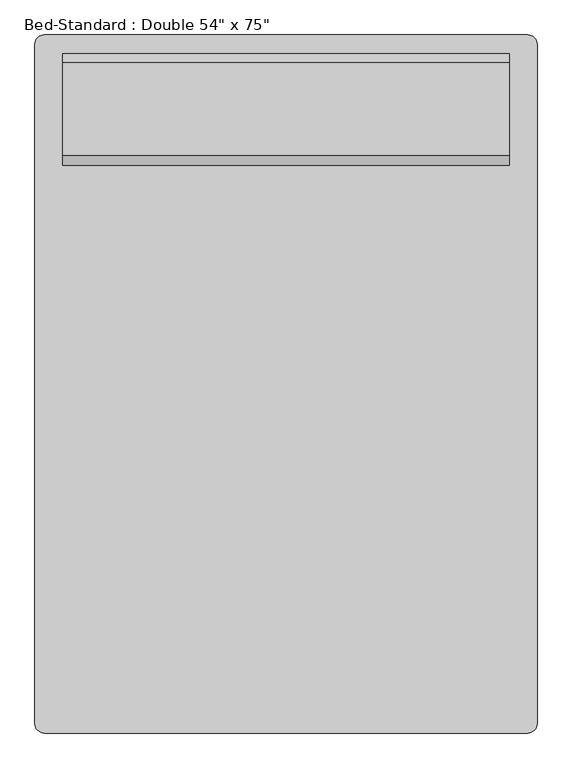
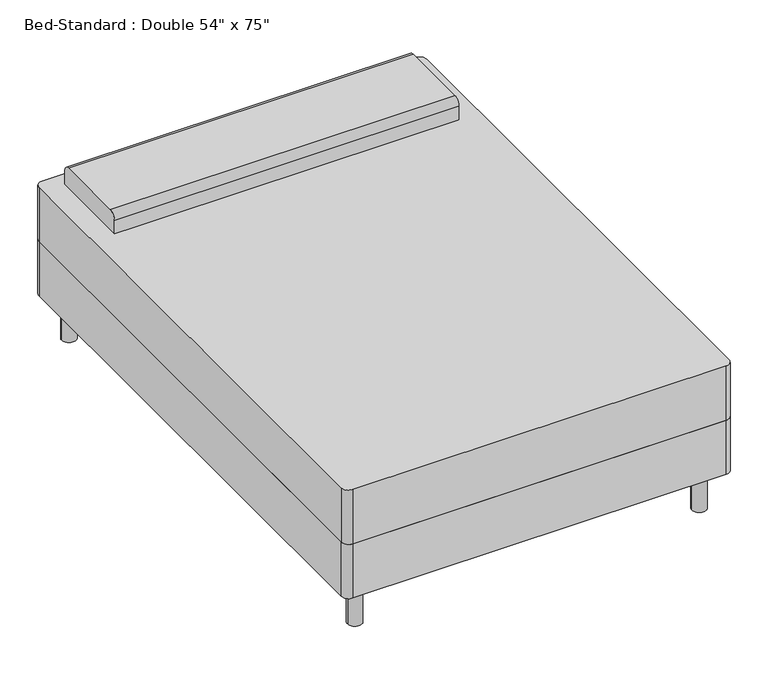
"""IFC4 building model written with IfcOpenShell, lengths in millimetres: furniture geometry."""

from ifc_helpers import new_model, si_unit, point, frame, frame_2d, origin, origin_with_axes, place, context, project, spatial, polyline, circle_curve, trimmed, segment, composite_curve, outline, extrude, source, transform, mapped, element, save


def furniture_52ef1662(model_context):
    return source(origin(), model_context, "Body", "SweptSolid", [
        extrude(outline(composite_curve([segment(polyline([(-388.9114754, 906.904918), (931.8885246, 906.904918)]), True, "CONTINUOUS"), segment(trimmed(circle_curve(frame_2d((931.8885246, 881.504918)), 25.4), [point((931.8885246, 906.904918))], [point((957.2885246, 881.504918))], False, "CARTESIAN"), True, "CONTINUOUS"), segment(polyline([(957.2885246, 881.504918), (957.2885246, -972.695082)]), True, "CONTINUOUS"), segment(trimmed(circle_curve(frame_2d((931.8885246, -972.695082)), 25.4), [point((957.2885246, -972.695082))], [point((931.8885246, -998.095082))], False, "CARTESIAN"), True, "CONTINUOUS"), segment(polyline([(931.8885246, -998.095082), (-388.9114754, -998.095082)]), True, "CONTINUOUS"), segment(trimmed(circle_curve(frame_2d((-388.9114754, -972.695082)), 25.4), [point((-388.9114754, -998.095082))], [point((-414.3114754, -972.695082))], False, "CARTESIAN"), True, "CONTINUOUS"), segment(polyline([(-414.3114754, -972.695082), (-414.3114754, 881.504918)]), True, "CONTINUOUS"), segment(trimmed(circle_curve(frame_2d((-388.9114754, 881.504918)), 25.4), [point((-414.3114754, 881.504918))], [point((-388.9114754, 906.904918))], False, "CARTESIAN"), True, "CONTINUOUS")], self_intersect=False)), frame((0.0, 0.0, 355.6), z_axis=(0.0, 0.0, 1.0), x_axis=(1.0, 0.0, 0.0)), (0.0, 0.0, 1.0), 203.2),
        extrude(outline(composite_curve([segment(trimmed(circle_curve(frame_2d((-338.1114754, 830.704918)), 25.4), [point((-363.5114754, 830.704918))], [point((-312.7114754, 830.704918))], False, "CARTESIAN"), True, "CONTINUOUS"), segment(trimmed(circle_curve(frame_2d((-338.1114754, 830.704918)), 25.4), [point((-312.7114754, 830.704918))], [point((-363.5114754, 830.704918))], False, "CARTESIAN"), True, "CONTINUOUS")], self_intersect=False)), origin_with_axes(), (0.0, 0.0, 1.0), 152.4),
        extrude(outline(composite_curve([segment(trimmed(circle_curve(frame_2d((881.0885246, 830.704918)), 25.4), [point((855.6885246, 830.704918))], [point((906.4885246, 830.704918))], False, "CARTESIAN"), True, "CONTINUOUS"), segment(trimmed(circle_curve(frame_2d((881.0885246, 830.704918)), 25.4), [point((906.4885246, 830.704918))], [point((855.6885246, 830.704918))], False, "CARTESIAN"), True, "CONTINUOUS")], self_intersect=False)), origin_with_axes(), (0.0, 0.0, 1.0), 152.4),
        extrude(outline(composite_curve([segment(trimmed(circle_curve(frame_2d((881.0885246, -921.895082)), 25.4), [point((855.6885246, -921.895082))], [point((906.4885246, -921.895082))], False, "CARTESIAN"), True, "CONTINUOUS"), segment(trimmed(circle_curve(frame_2d((881.0885246, -921.895082)), 25.4), [point((906.4885246, -921.895082))], [point((855.6885246, -921.895082))], False, "CARTESIAN"), True, "CONTINUOUS")], self_intersect=False)), origin_with_axes(), (0.0, 0.0, 1.0), 152.4),
        extrude(outline(composite_curve([segment(trimmed(circle_curve(frame_2d((-338.1114754, -921.895082)), 25.4), [point((-363.5114754, -921.895082))], [point((-312.7114754, -921.895082))], False, "CARTESIAN"), True, "CONTINUOUS"), segment(trimmed(circle_curve(frame_2d((-338.1114754, -921.895082)), 25.4), [point((-312.7114754, -921.895082))], [point((-363.5114754, -921.895082))], False, "CARTESIAN"), True, "CONTINUOUS")], self_intersect=False)), origin_with_axes(), (0.0, 0.0, 1.0), 152.4),
        extrude(outline(composite_curve([segment(polyline([(551.304918, 558.8), (551.304918, 609.6)]), True, "CONTINUOUS"), segment(trimmed(circle_curve(frame_2d((576.704918, 609.6)), 25.4), [point((551.304918, 609.6))], [point((576.704918, 635.0))], False, "CARTESIAN"), True, "CONTINUOUS"), segment(polyline([(576.704918, 635.0), (830.704918, 635.0)]), True, "CONTINUOUS"), segment(trimmed(circle_curve(frame_2d((830.704918, 609.6)), 25.4), [point((830.704918, 635.0))], [point((856.104918, 609.6))], False, "CARTESIAN"), True, "CONTINUOUS"), segment(polyline([(856.104918, 609.6), (856.104918, 558.8), (551.304918, 558.8)]), True, "CONTINUOUS")], self_intersect=False)), frame((-338.1114754, 0.0, 0.0), z_axis=(1.0, 0.0, 0.0), x_axis=(0.0, 1.0, 0.0)), (0.0, 0.0, 1.0), 1219.2),
        extrude(outline(composite_curve([segment(polyline([(-414.3114754, -972.695082), (-414.3114754, 881.504918)]), True, "CONTINUOUS"), segment(trimmed(circle_curve(frame_2d((-388.9114754, 881.504918)), 25.4), [point((-414.3114754, 881.504918))], [point((-388.9114754, 906.904918))], False, "CARTESIAN"), True, "CONTINUOUS"), segment(polyline([(-388.9114754, 906.904918), (931.8885246, 906.904918)]), True, "CONTINUOUS"), segment(trimmed(circle_curve(frame_2d((931.8885246, 881.504918)), 25.4), [point((931.8885246, 906.904918))], [point((957.2885246, 881.504918))], False, "CARTESIAN"), True, "CONTINUOUS"), segment(polyline([(957.2885246, 881.504918), (957.2885246, -972.695082)]), True, "CONTINUOUS"), segment(trimmed(circle_curve(frame_2d((931.8885246, -972.695082)), 25.4), [point((957.2885246, -972.695082))], [point((931.8885246, -998.095082))], False, "CARTESIAN"), True, "CONTINUOUS"), segment(polyline([(931.8885246, -998.095082), (-388.9114754, -998.095082)]), True, "CONTINUOUS"), segment(trimmed(circle_curve(frame_2d((-388.9114754, -972.695082)), 25.4), [point((-388.9114754, -998.095082))], [point((-414.3114754, -972.695082))], False, "CARTESIAN"), True, "CONTINUOUS")], self_intersect=False)), frame((0.0, 0.0, 152.4), z_axis=(0.0, 0.0, 1.0), x_axis=(1.0, 0.0, 0.0)), (0.0, 0.0, 1.0), 203.2),
    ])


if __name__ == "__main__":
    model = new_model("IFC4")
    model_context = context("Model", 3, world=origin())
    ifc_project = project(units=[si_unit("LENGTHUNIT", "METRE", prefix="MILLI")], contexts=[model_context])
    site = spatial("IfcSite", under=ifc_project)
    building = spatial("IfcBuilding", under=site)
    placement = place(None, origin())
    furniture_shape = furniture_52ef1662(model_context)
    element("IfcFurniture", 1, ObjectType="Bed-Standard : Double 54\" x 75\"", at=placement, inside=building, context=model_context, shape_type="MappedRepresentation", body=[
        mapped(furniture_shape, transform((0.0, 0.0, 0.0), x_axis=(1.0, 0.0, 0.0), y_axis=(0.0, 1.0, 0.0), z_axis=(0.0, 0.0, 1.0))),
    ])
    save(model, "model.ifc")

# Revit data of these elements
# Type "Bed-Standard : Double 54\" x 75\""
#   Assembly Code = "E2020200"
#   Length = 6' - 3"
#   Width = 4' - 6"
#   Leg Material = Steel, Chrome Plated
#   Mattress Material = Linen, White
#   Default Elevation = 0
# Element 1 (IfcFurniture, "Bed-Standard : Double 54\" x 75\"")
#   Materials on its faces: "Linen, White", "Steel, Chrome Plated"
# Materials
#   "Steel, Chrome Plated": class "Metal", colour RGB 17 17 17, transparency 0, Description = "Chromiuim plated steel", Cost = 0
#   "Linen, White": class "Textile", colour RGB 206 206 206, transparency 0, Description = "Linen, white", Cost = 0
